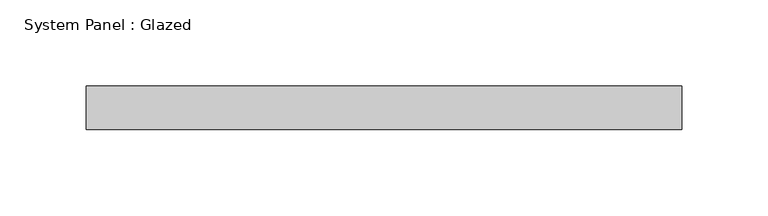
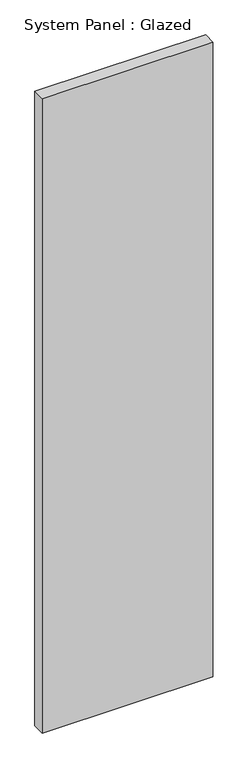
"""IFC4 building model written with IfcOpenShell, lengths in millimetres: plate geometry, System Panel : Glazed."""

from ifc_helpers import new_model, si_unit, origin, origin_with_axes, place, context, project, spatial, polyline, outline, extrude, source, transform, mapped, element, save


def system_panel_glazed_7b9e2e16(model_context):
    return source(origin(), model_context, "Body", "SweptSolid", [
        extrude(outline(polyline([(173.0375, 19.05), (-173.0375, 19.05), (-173.0375, 44.45), (173.0375, 44.45), (173.0375, 19.05)])), origin_with_axes(), (0.0, 0.0, 1.0), 1359.9744191),
    ])


if __name__ == "__main__":
    model = new_model("IFC4")
    model_context = context("Model", 3, world=origin())
    ifc_project = project(units=[si_unit("LENGTHUNIT", "METRE", prefix="MILLI")], contexts=[model_context])
    site = spatial("IfcSite", under=ifc_project)
    building = spatial("IfcBuilding", under=site)
    placement = place(None, origin())
    system_panel_glazed_shape = system_panel_glazed_7b9e2e16(model_context)
    element("IfcPlate", 1, ObjectType="System Panel : Glazed", at=placement, inside=building, context=model_context, shape_type="MappedRepresentation", body=[
        mapped(system_panel_glazed_shape, transform((0.0, 0.0, 0.0), x_axis=(1.0, 0.0, 0.0), y_axis=(0.0, 1.0, 0.0), z_axis=(0.0, 0.0, 1.0))),
    ])
    save(model, "model.ifc")

# Revit data of these elements
# Type "System Panel : Glazed"
#   Construction Type Id = "GSP4R"
#   Analytic Construction = "1/8 in Pilkington single glazing"
#   Visual Light Transmittance = 0.9
#   Solar Heat Gain Coefficient = 0.86
#   Heat Transfer Coefficient (U) = 1.18115 BTU/(h·ft²·°F)
#   Define Thermal Properties by = 1
# Element 1 (IfcPlate, "System Panel : Glazed")
#   Materials on its faces: "Glass"
# Materials
#   "Glass": class "Glass", colour RGB 0 128 192, transparency 0.75, Description = "Soda Lime Glass", Cost = 0
